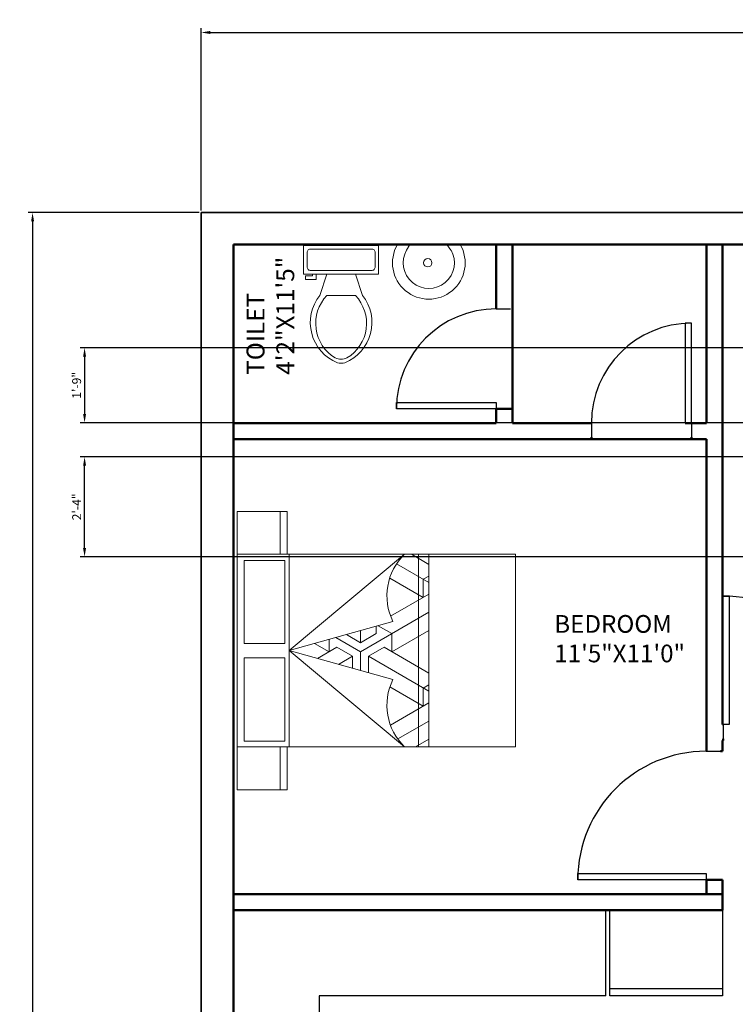
# Model space of a CAD drawing. Units: inches. Extents: x 1455 to 2044, y 1728 to 2439.
# Tile 3 of 4: x 1455 to 1655, y 2128 to 2404. Entities that reach past the tile are written whole.
import ezdxf

# ---------------------------------------------------------------- set-up
doc = ezdxf.new("R2010")
doc.units = ezdxf.units.IN
for name, color, linetype, lineweight in [('A-ANNO-DIMS', 2, 'Continuous', 18), ('A-AREA-IDEN', 7, 'Continuous', 25), ('A-DOOR', 4, 'Continuous', 25), ('A-FLOR-CASE', 8, 'Continuous', 25), ('A-FLOR-FIXT', 9, 'Continuous', 18), ('A-FURN', 8, 'Continuous', 18), ('A-WALL', 7, 'Continuous', 50), ('C-PROP', 7, 'Continuous', 35)]:
    doc.layers.add(name, color=color, linetype=linetype, lineweight=lineweight)
doc.styles.get("Standard").update_dxf_attribs({"font": 'arial.ttf'})
doc.dimstyles.new('ISO-25', dxfattribs={"dimtxt": 2.5, "dimasz": 2.5, "dimexe": 1.25, "dimexo": 0.625, "dimtad": 1, "dimlunit": 3, "dimtxsty": 'Standard', "dimcen": 2.5, "dimadec": 0, "dimazin": 0, "dimtfac": 1, "dimtmove": 0, "dimatfit": 3, "dimfxl": 1, "dimarcsym": 0})

# ---------------------------------------------------------------- blocks, each defined once
blk = doc.blocks.new('*U2')
for p, q in [((9.5, -6), (9.5, -2)), ((-8, -8.5), (-8, -8)), ((-7, -8), (-7, -9.5)), ((-4, -8), (-6, -14)), ((4, -8), (6, -14)), ((-10, -8.5), (-8, -8.5)), ((-10, -9.5), (-10, -8.5)), ((-7, -9.5), (-10, -9.5)), ((4, -14), (-4, -14))]:
    blk.add_line(p, q)
blk.add_lwpolyline([(10.5, -8), (10.5, 0), (-10.5, 0), (-10.5, -8)], close=True)
for points in [[(-9.5, -2), (-9.5, -6)], [(8.5, -1), (-8.5, -1)], [(-8.5, -7), (8.5, -7)]]:
    blk.add_lwpolyline(points)
for centre, radius, start, end in [((-8.62, -1.88), 0.884, 81.8699, 188.1301), ((8.62, -1.88), 0.884, 351.8699, 98.1301), ((-8.62, -6.12), 0.884, 171.8699, 278.1301), ((8.62, -6.12), 0.884, 261.8699, 8.1301), ((3.52, -21.58), 12.17, 141.4691, 247.9714), ((4.2, -21.82), 11.33, 136.3677, 238.9468), ((-3.52, -21.58), 12.17, 292.0284, 38.5307), ((-4.2, -21.82), 11.33, 301.053, 43.6321), ((0, -27.88), 4, 245.7318, 294.2682), ((0, -29), 4, 254.8605, 285.1395)]:
    blk.add_arc(centre, radius, start, end)
blk = doc.blocks.new('*U4')
for p, q in [((-28, 0), (-28, -4)), ((0, 0), (0, -4))]:
    blk.add_line(p, q)
blk.add_lwpolyline([(0, 0), (0, 28), (-1.75, 28), (-1.75, 0)], close=True)
blk.add_arc((0, 0), 28, 90, 180)
blk = doc.blocks.new('*U5')
for p, q in [((0, 0), (0, -4)), ((28, 0), (28, -4))]:
    blk.add_line(p, q)
blk.add_lwpolyline([(0, 0), (0, 28), (1.75, 28), (1.75, 0)], close=True)
blk.add_arc((0, 0), 28, 0, 90)
blk = doc.blocks.new('*U6')
for p, q in [((-36, 0), (-36, 4)), ((0, 0), (0, 4))]:
    blk.add_line(p, q)
blk.add_lwpolyline([(0, 0), (0, -36), (-1.75, -36), (-1.75, 0)], close=True)
blk.add_arc((0, 0), 36, 180, 270)
blk = doc.blocks.new('*U7')
for p, q in [((0, 0), (0, -4)), ((36, 0), (36, -4))]:
    blk.add_line(p, q)
blk.add_lwpolyline([(0, 0), (0, 36), (1.75, 36), (1.75, 0)], close=True)
blk.add_arc((0, 0), 36, 0, 90)
blk = doc.blocks.new('*D16')
at = {"layer": 'A-ANNO-DIMS', "color": 0, "lineweight": -2, "transparency": 16777216}
for p, q in [((1504.95, 2349.58), (1457.06, 2349.58)), ((1458.31, 2347.08), (1458.31, 1764.08)), ((1504.95, 1761.58), (1457.06, 1761.58))]:
    blk.add_line(p, q, dxfattribs=at)
at = {"layer": 'A-ANNO-DIMS', "color": 0, "transparency": 16777216}
for points in [[(1457.9, 2347.08), (1458.73, 2347.08), (1458.31, 2349.58)], [(1457.9, 1764.08), (1458.73, 1764.08), (1458.31, 1761.58)]]:
    blk.add_solid(points, dxfattribs=at)
at = {"layer": 'Defpoints', "color": 0, "transparency": 16777216}
for p in [(1505.58, 2349.58), (1458.31, 1761.58), (1505.58, 1761.58)]:
    blk.add_point(p, dxfattribs=at)
at = {"layer": 'A-ANNO-DIMS', "color": 0, "transparency": 16777216, "insert": (1456.41, 2055.58), "char_height": 2.5, "attachment_point": 5, "rotation": 90}
blk.add_mtext("49'", dxfattribs=at)
blk = doc.blocks.new('*D17')
at = {"layer": 'A-ANNO-DIMS', "color": 0, "lineweight": -2, "transparency": 16777216}
for p, q in [((1505.58, 2350.2), (1505.58, 2401.3)), ((2009.58, 2350.2), (2009.58, 2401.3)), ((1508.08, 2400.05), (2007.08, 2400.05))]:
    blk.add_line(p, q, dxfattribs=at)
at = {"layer": 'A-ANNO-DIMS', "color": 0, "transparency": 16777216}
for points in [[(1508.08, 2400.47), (1508.08, 2399.63), (1505.58, 2400.05)], [(2007.08, 2400.47), (2007.08, 2399.63), (2009.58, 2400.05)]]:
    blk.add_solid(points, dxfattribs=at)
at = {"layer": 'Defpoints', "color": 0, "transparency": 16777216}
for p in [(2009.58, 2400.05), (1505.58, 2349.58), (2009.58, 2349.58)]:
    blk.add_point(p, dxfattribs=at)
at = {"layer": 'A-ANNO-DIMS', "color": 0, "transparency": 16777216, "insert": (1757.58, 2401.93), "char_height": 2.5, "attachment_point": 5}
blk.add_mtext("42'", dxfattribs=at)
blk = doc.blocks.new('BED-DOUBLE-WITH-NIGHTSTANDS')
h = blk.add_hatch()
h.set_pattern_fill('ESCHER', color=256, angle=-270)
h.set_pattern_definition([(150, (2210.078, -2055.985), (7e-09, -30.48), [27.94, -2.54]), (270, (2210.078, -2055.985), (26.39645, 15.24), [27.94, -2.54]), (30, (2210.078, -2055.985), (7e-09, 30.48), [27.94, -2.54]), (150, (2210.078, -2053.445), (7e-09, -30.48), [5.08, -25.4]), (30, (2210.078, -2053.445), (7e-09, 30.48), [5.08, -25.4]), (150, (2207.88, -2057.255), (7e-09, -30.48), [5.08, -25.4]), (270, (2207.88, -2057.255), (26.39645, 15.24), [5.08, -25.4]), (30, (2212.278, -2057.255), (7e-09, 30.48), [5.08, -25.4]), (270, (2212.278, -2057.255), (26.39645, 15.24), [5.08, -25.4]), (150, (2210.078, -2066.145), (7e-09, -30.48), [5.08, -25.4]), (30, (2210.078, -2066.145), (7e-09, 30.48), [5.08, -25.4]), (150, (2218.877, -2050.905), (7e-09, -30.48), [5.08, -25.4]), (270, (2218.877, -2050.905), (26.39645, 15.24), [5.08, -25.4]), (30, (2201.28, -2050.905), (7e-09, 30.48), [5.08, -25.4]), (270, (2201.28, -2050.905), (26.39645, 15.24), [5.08, -25.4]), (90, (2205.68, -2050.905), (-26.39645, -15.24), [17.78, -12.7]), (90, (2214.478, -2050.905), (-26.39645, -15.24), [17.78, -12.7]), (210, (2203.48, -2054.715), (-7e-09, -30.48), [17.78, -12.7]), (210, (2207.88, -2062.335), (-7e-09, -30.48), [17.78, -12.7]), (330, (2212.278, -2062.335), (26.39645, 15.24), [17.78, -12.7]), (330, (2216.678, -2054.715), (26.39645, 15.24), [17.78, -12.7])])
h.paths.add_polyline_path([(-31.09, 54, 0.326433), (-34.36, 35.12), (-63.46, 27), (-34.36, 18.88, 0.326433), (-31.09, 0), (-27.21, 0), (-27.21, 54)])
h.paths.add_polyline_path([(-27.21, 54), (-27.21, 0), (-24.3, 0), (-24.3, 54)])
for p, q in [((-78, 54), (-78, 66)), ((-78, 66), (-66, 66)), ((-66, 66), (-66, 54)), ((-66, 66), (-64, 66)), ((-64, 66), (-64, 54)), ((-63.46, 0), (-63.46, 54)), ((-63.46, 27), (-31.09, 54)), ((-63.46, 27), (-34.36, 35.12)), ((-76.01, 28.95), (-64.69, 28.95)), ((-76.01, 24.95), (-64.69, 24.95)), ((-63.46, 27), (-31.09, 0)), ((-63.46, 27), (-34.36, 18.88)), ((-78, 0), (-78, -12)), ((-66, -12), (-66, 0)), ((-64, -12), (-64, 0)), ((-78, -12), (-66, -12)), ((-66, -12), (-64, -12))]:
    blk.add_line(p, q)
for points in [[(0, 0), (0, 54), (-78, 54), (-78, 0)], [(-27.21, 0), (-27.21, 54), (-24.3, 54), (-24.3, 0)]]:
    blk.add_lwpolyline(points, close=True)
for points in [[(-76.01, 28.95), (-76.01, 52.28), (-64.69, 52.28), (-64.69, 28.95)], [(-64.69, 24.95), (-64.69, 1.63), (-76.01, 1.63), (-76.01, 24.95)]]:
    blk.add_lwpolyline(points)
for centre, start, end in [((-19.81, 42.32), 134.0109, 206.3245), ((-19.81, 11.68), 153.6755, 225.9891)]:
    blk.add_arc(centre, 16.24, start, end)
blk = doc.blocks.new('BASIN-WALL-MOUNT')
for p, q in [((-6.21, 3.6), (-5.3, 5.1)), ((6.21, 3.6), (5.05, 5.1))]:
    blk.add_line(p, q)
blk.add_circle((-0.29, 0.03), 1.16)
for radius in [10.18, 7.18]:
    blk.add_arc((0, 0), radius, 149.9376, 30.0624)
blk = doc.blocks.new('*D37')
at = {"layer": 'A-ANNO-DIMS', "color": 0, "lineweight": -2, "transparency": 16777216}
for p, q in [((1792.95, 2281.09), (1471.63, 2281.09)), ((1472.88, 2255.58), (1472.88, 2278.59)), ((1792.95, 2253.08), (1471.63, 2253.08))]:
    blk.add_line(p, q, dxfattribs=at)
at = {"layer": 'A-ANNO-DIMS', "color": 0, "transparency": 16777216}
for points in [[(1472.46, 2278.59), (1473.3, 2278.59), (1472.88, 2281.09)], [(1472.46, 2255.58), (1473.3, 2255.58), (1472.88, 2253.08)]]:
    blk.add_solid(points, dxfattribs=at)
at = {"layer": 'Defpoints', "color": 0, "transparency": 16777216}
for p in [(1472.88, 2281.09), (1793.58, 2281.09), (1793.58, 2253.08)]:
    blk.add_point(p, dxfattribs=at)
at = {"layer": 'A-ANNO-DIMS', "color": 0, "transparency": 16777216, "insert": (1471, 2267.09), "char_height": 2.5, "attachment_point": 5, "rotation": 90}
blk.add_mtext('2\'-4"', dxfattribs=at)
blk = doc.blocks.new('*D42')
at = {"layer": 'A-ANNO-DIMS', "color": 0, "lineweight": -2, "transparency": 16777216}
for p, q in [((1838.65, 2311.66), (1471.63, 2311.66)), ((1472.88, 2309.16), (1472.88, 2293.16)), ((1838.65, 2290.66), (1471.63, 2290.66))]:
    blk.add_line(p, q, dxfattribs=at)
at = {"layer": 'A-ANNO-DIMS', "color": 0, "transparency": 16777216}
for points in [[(1472.46, 2309.16), (1473.3, 2309.16), (1472.88, 2311.66)], [(1472.46, 2293.16), (1473.3, 2293.16), (1472.88, 2290.66)]]:
    blk.add_solid(points, dxfattribs=at)
at = {"layer": 'Defpoints', "color": 0, "transparency": 16777216}
for p in [(1839.27, 2311.66), (1472.88, 2290.66), (1839.27, 2290.66)]:
    blk.add_point(p, dxfattribs=at)
at = {"layer": 'A-ANNO-DIMS', "color": 0, "transparency": 16777216, "insert": (1470.98, 2301.16), "char_height": 2.5, "attachment_point": 5, "rotation": 90}
blk.add_mtext('1\'-9"', dxfattribs=at)

msp = doc.modelspace()

# ---------------------------------------------------------------- linework, layer by layer
at = {"layer": 'A-FLOR-CASE'}
for p, q in [((1620.07, 2130.079), (1620.07, 2154.079)), ((1651.58, 2154.079), (1651.58, 2130.079)), ((1620.07, 2132.123), (1651.58, 2132.123)), ((1514.58, 2130.055), (1514.58, 2038.579)), ((1618.882, 2130.055), (1538.58, 2130.055)), ((1538.58, 2130.055), (1538.58, 2062.579)), ((1627.58, 2130.079), (1620.07, 2130.079)), ((1651.58, 2130.079), (1627.58, 2130.079))]:
    msp.add_line(p, q, dxfattribs=at)
for points in [[(1618.882, 2130.055), (1618.882, 2154.079), (1642.882, 2154.079)], [(1642.882, 2130.079), (1642.882, 2130.055)]]:
    msp.add_lwpolyline(points, dxfattribs=at)
at = {"layer": 'A-WALL'}
for p, q in [((1514.58, 2340.579), (2000.58, 2340.579)), ((1514.58, 1998.079), (1514.58, 2340.579)), ((1588.225, 2322.578), (1588.225, 2340.579)), ((1592.725, 2294.579), (1592.725, 2340.579)), ((1647.08, 2290.579), (1647.08, 2340.579)), ((1651.58, 2206.079), (1651.58, 2340.579)), ((1588.225, 2290.579), (1588.225, 2294.579)), ((1588.225, 2294.579), (1592.725, 2294.579)), ((1592.725, 2294.579), (1592.725, 2290.579)), ((1514.58, 2290.579), (1588.225, 2290.579)), ((1592.725, 2290.579), (1614.892, 2290.579)), ((1641.142, 2290.579), (1647.08, 2290.579)), ((1647.08, 2290.579), (1643.08, 2290.579)), ((1514.58, 2286.079), (1647.08, 2286.079)), ((1614.892, 2286.579), (1614.892, 2286.079)), ((1642.892, 2286.579), (1642.892, 2286.079)), ((1647.08, 2201.579), (1647.08, 2286.079)), ((1651.58, 2206.079), (1651.746, 2206.079)), ((1647.08, 2201.579), (1647.08, 2198.597)), ((1651.58, 2201.579), (1651.746, 2201.579)), ((1651.58, 2201.579), (1651.58, 2198.597)), ((1651.746, 2202.084), (1651.746, 2201.579)), ((1651.058, 2198.597), (1651.58, 2198.597)), ((1647.058, 2163.472), (1647.058, 2163.472)), ((1651.58, 2162.579), (1647.08, 2162.579)), ((1647.08, 2162.579), (1647.08, 2158.579)), ((1651.58, 2158.579), (1651.58, 2162.579)), ((1514.58, 2158.579), (1647.08, 2158.579)), ((1647.08, 2158.579), (1651.58, 2158.579)), ((1651.58, 2154.079), (1651.58, 2158.579)), ((1514.58, 2154.079), (1647.08, 2154.079)), ((1647.08, 2154.079), (1651.58, 2154.079))]:
    msp.add_line(p, q, dxfattribs=at)
at = {"layer": 'C-PROP'}
for p, q in [((1505.58, 2349.579), (2009.58, 2349.579)), ((1505.58, 1761.579), (1505.58, 2349.579))]:
    msp.add_line(p, q, dxfattribs=at)

# ---------------------------------------------------------------- block references
at = {"layer": 'A-DOOR'}
for name, p, rotation in [('*U5', (1588.225, 2294.578), 90), ('*U6', (1647.058, 2162.597), 270)]:
    msp.add_blockref(name, p, dxfattribs=dict(at, rotation=rotation))
for name, p in [('*U4', (1642.892, 2290.579)), ('*U7', (1651.746, 2206.084))]:
    msp.add_blockref(name, p, dxfattribs=at)
at = {"layer": 'A-FLOR-FIXT'}
for name, p in [('*U2', (1544.758, 2340.346)), ('BASIN-WALL-MOUNT', (1569.328, 2335.48))]:
    msp.add_blockref(name, p, dxfattribs=at)
at = {"layer": 'A-FURN'}
msp.add_blockref('BED-DOUBLE-WITH-NIGHTSTANDS', (1593.635, 2199.811), dxfattribs=at)

# ---------------------------------------------------------------- texts
at = {"layer": 'A-AREA-IDEN', "insert": (1518.28, 2304.097), "char_height": 5, "attachment_point": 1, "rotation": 90}
msp.add_mtext_dynamic_manual_height_columns('TOILET\\P4\'2"X11\'5"', width=11.65064, gutter_width=25, heights=[0], dxfattribs=at)
at = {"layer": 'A-AREA-IDEN', "insert": (1604.47, 2236.763), "char_height": 4.96644, "attachment_point": 1}
msp.add_mtext_dynamic_manual_height_columns('BEDROOM \\P11\'5"X11\'0"', width=79.74969, gutter_width=24.832, heights=[0], dxfattribs=at)

# ---------------------------------------------------------------- dimensions: what is measured, and where the dimension line sits
at = {"layer": 'A-ANNO-DIMS'}
dim = msp.add_linear_dim(base=(2009.58, 2400.051), p1=(1505.58, 2349.579), p2=(2009.58, 2349.579), dimstyle='ISO-25', override={"dimclrd": 0, "dimclre": 0, "dimclrt": 0}, dxfattribs=at)
dim.commit()
dim.dimension.update_dxf_attribs({"geometry": '*D17', "text_midpoint": (1757.58, 2401.931)})
for base, p1, p2, override, picture, middle in [((1458.313, 1761.579), (1505.58, 2349.579), (1505.58, 1761.579), {"dimclrd": 0, "dimclre": 0, "dimclrt": 0}, '*D16', (1456.412, 2055.579)), ((1472.88, 2290.665), (1839.271, 2311.665), (1839.271, 2290.665), {"dimdec": 1, "dimlfac": 1, "dimrnd": 0, "dimzin": 1, "dimdsep": 46, "dimlunit": 4, "dimfrac": 2}, '*D42', (1470.978, 2301.165)), ((1472.88, 2281.092), (1793.58, 2253.079), (1793.58, 2281.092), {"dimdec": 1, "dimlfac": 1, "dimrnd": 0, "dimzin": 1, "dimdsep": 46, "dimlunit": 4, "dimfrac": 2}, '*D37', (1470.999, 2267.086))]:
    dim = msp.add_linear_dim(base=base, p1=p1, p2=p2, angle=90, dimstyle='ISO-25', override=override, dxfattribs=at)
    dim.commit()
    dim.dimension.update_dxf_attribs({"geometry": picture, "text_midpoint": middle})

doc.saveas('drawing.dxf')
